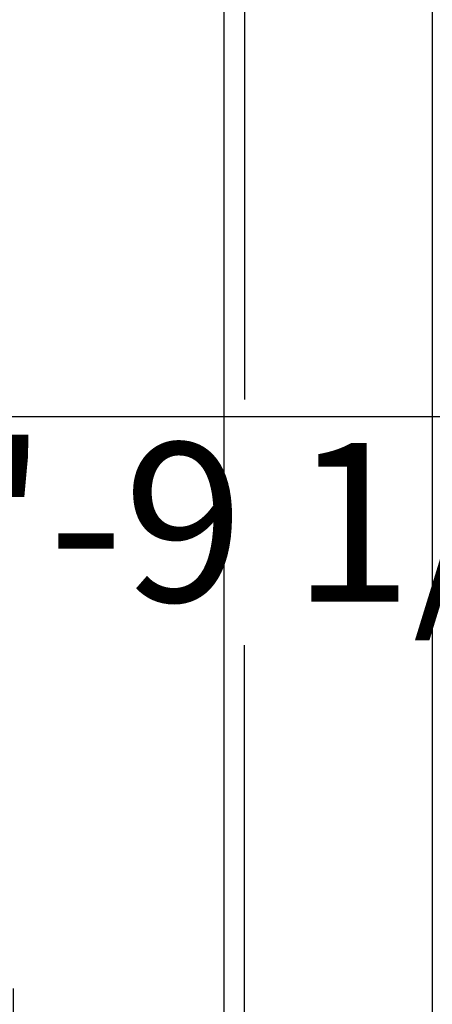
# Model space of a CAD drawing. Units: inches. Extents: x -26 to 385, y 12 to 697.
# Tile 8 of 13: x 264 to 285, y 165 to 215. Entities that reach past the tile are written whole.
import ezdxf

# ---------------------------------------------------------------- set-up
doc = ezdxf.new("R2010")
doc.units = ezdxf.units.IN
doc.header["$MEASUREMENT"] = 0
doc.layers.add('A-ANNO-DIMS', color=4, linetype='Continuous', lineweight=18)
doc.styles.get("Standard").update_dxf_attribs({"font": 'italic8.shx'})
doc.dimstyles.get("Standard").update_dxf_attribs({"dimtxt": 8, "dimasz": 0.18, "dimexe": 0.18, "dimexo": 0.0625, "dimgap": 0.09, "dimtad": 0, "dimtih": 1, "dimtoh": 1, "dimdec": 4, "dimzin": 0, "dimdsep": 46, "dimlunit": 3, "dimtxsty": 'Standard', "dimcen": 0.09, "dimclrd": 2, "dimclre": 3, "dimclrt": 6, "dimadec": 0, "dimazin": 0, "dimtfac": 1, "dimtdec": 4, "dimtofl": 0, "dimtmove": 0, "dimatfit": 3, "dimfxl": 1, "dimtolj": 1, "dimtzin": 0, "dimarcsym": 0})

# ---------------------------------------------------------------- blocks, each defined once
blk = doc.blocks.new('*D11')
at = {"layer": 'A-ANNO-DIMS', "color": 3, "lineweight": -2, "transparency": 16777216}
for p, q in [((285.56, 224.402), (274.992, 224.402)), ((285.56, 154.738), (274.992, 154.738))]:
    blk.add_line(p, q, dxfattribs=at)
at = {"layer": 'A-ANNO-DIMS', "color": 2, "lineweight": -2, "transparency": 16777216}
for p, q in [((275.172, 224.222), (275.172, 195.755)), ((275.172, 154.918), (275.172, 183.384))]:
    blk.add_line(p, q, dxfattribs=at)
at = {"layer": 'A-ANNO-DIMS', "color": 2, "transparency": 16777216}
for points in [[(275.142, 224.222), (275.202, 224.222), (275.172, 224.402)], [(275.142, 154.918), (275.202, 154.918), (275.172, 154.738)]]:
    blk.add_solid(points, dxfattribs=at)
at = {"layer": 'Defpoints', "color": 0, "transparency": 16777216}
for p in [(285.622, 224.402), (275.172, 154.738), (285.622, 154.738)]:
    blk.add_point(p, dxfattribs=at)
at = {"layer": 'A-ANNO-DIMS', "color": 6, "transparency": 16777216, "insert": (275.172, 189.57), "char_height": 8, "attachment_point": 5}
blk.add_mtext('\\A1;SOFA 5\'-9 1/2" TYP.', dxfattribs=at)
blk = doc.blocks.new('*D25')
at = {"layer": 'A-ANNO-DIMS', "color": 3, "lineweight": -2, "transparency": 16777216}
for p, q in [((284.629322, 368.316588), (284.629322, 23.949088)), ((320.629322, 368.316588), (320.629322, 23.949088))]:
    blk.add_line(p, q, dxfattribs=at)
at = {"layer": 'A-ANNO-DIMS', "color": 2, "lineweight": -2, "transparency": 16777216}
for p, q in [((284.449322, 24.129088), (284.269322, 24.129088)), ((320.809322, 24.129088), (320.989322, 24.129088))]:
    blk.add_line(p, q, dxfattribs=at)
at = {"layer": 'A-ANNO-DIMS', "color": 2, "transparency": 16777216}
for points in [[(284.449322, 24.159088), (284.449322, 24.099088), (284.629322, 24.129088)], [(320.809322, 24.159088), (320.809322, 24.099088), (320.629322, 24.129088)]]:
    blk.add_solid(points, dxfattribs=at)
at = {"layer": 'Defpoints', "color": 0, "transparency": 16777216}
for p in [(284.629322, 368.379088), (320.629322, 368.379088), (320.629322, 24.129088)]:
    blk.add_point(p, dxfattribs=at)
at = {"layer": 'A-ANNO-DIMS', "color": 6, "transparency": 16777216, "insert": (302.629322, 24.129088), "char_height": 8, "attachment_point": 5}
blk.add_mtext('\\A1;3\'-0"', dxfattribs=at)
blk = doc.blocks.new('*D28')
at = {"layer": 'A-ANNO-DIMS', "color": 3, "lineweight": -2, "transparency": 16777216}
for p, q in [((141.692, 194.903), (355.559, 194.903)), ((141.692, 158.903), (355.559, 158.903))]:
    blk.add_line(p, q, dxfattribs=at)
at = {"layer": 'A-ANNO-DIMS', "color": 2, "lineweight": -2, "transparency": 16777216}
for p, q in [((355.379, 194.723), (355.379, 181.755)), ((355.379, 159.083), (355.379, 172.052))]:
    blk.add_line(p, q, dxfattribs=at)
at = {"layer": 'A-ANNO-DIMS', "color": 2, "transparency": 16777216}
for points in [[(355.349, 194.723), (355.409, 194.723), (355.379, 194.903)], [(355.349, 159.083), (355.409, 159.083), (355.379, 158.903)]]:
    blk.add_solid(points, dxfattribs=at)
at = {"layer": 'Defpoints', "color": 0, "transparency": 16777216}
for p in [(141.629, 194.903), (355.379, 194.903), (141.629, 158.903)]:
    blk.add_point(p, dxfattribs=at)
at = {"layer": 'A-ANNO-DIMS', "color": 6, "transparency": 16777216, "insert": (355.379, 176.903), "char_height": 8, "attachment_point": 5}
blk.add_mtext('\\A1;3\'-0"', dxfattribs=at)
blk = doc.blocks.new('*D31')
at = {"layer": 'A-ANNO-DIMS', "color": 3, "lineweight": -2, "transparency": 16777216}
for p, q in [((239.888, 166.079), (239.888, 23.949)), ((263.51, 166.079), (263.51, 23.949))]:
    blk.add_line(p, q, dxfattribs=at)
at = {"layer": 'A-ANNO-DIMS', "color": 2, "lineweight": -2, "transparency": 16777216}
for p, q in [((240.068, 24.129), (263.33, 24.129)), ((263.51, 24.129), (263.69, 24.129))]:
    blk.add_line(p, q, dxfattribs=at)
at = {"layer": 'A-ANNO-DIMS', "color": 2, "transparency": 16777216}
for points in [[(240.068, 24.159), (240.068, 24.099), (239.888, 24.129)], [(263.33, 24.159), (263.33, 24.099), (263.51, 24.129)]]:
    blk.add_solid(points, dxfattribs=at)
at = {"layer": 'Defpoints', "color": 0, "transparency": 16777216}
for p in [(239.888, 166.141), (263.51, 166.141), (263.51, 24.129)]:
    blk.add_point(p, dxfattribs=at)
at = {"layer": 'A-ANNO-DIMS', "color": 6, "transparency": 16777216, "insert": (296.732, 24.129), "char_height": 8, "attachment_point": 5}
blk.add_mtext('\\A1;1\'-11 1/2"', dxfattribs=at)
blk = doc.blocks.new('*D35')
at = {"layer": 'A-ANNO-DIMS', "color": 3, "lineweight": -2, "transparency": 16777216}
for p, q in [((193.598, 147.942), (193.598, 684.809)), ((244.986, 147.942), (244.986, 684.809))]:
    blk.add_line(p, q, dxfattribs=at)
at = {"layer": 'A-ANNO-DIMS', "color": 2, "lineweight": -2, "transparency": 16777216}
for p, q in [((193.778, 684.629), (244.806, 684.629)), ((244.986, 684.629), (245.166, 684.629))]:
    blk.add_line(p, q, dxfattribs=at)
at = {"layer": 'A-ANNO-DIMS', "color": 2, "transparency": 16777216}
for points in [[(193.778, 684.659), (193.778, 684.599), (193.598, 684.629)], [(244.806, 684.659), (244.806, 684.599), (244.986, 684.629)]]:
    blk.add_solid(points, dxfattribs=at)
at = {"layer": 'Defpoints', "color": 0, "transparency": 16777216}
for p in [(244.986, 684.629), (193.598, 147.879), (244.986, 147.879)]:
    blk.add_point(p, dxfattribs=at)
at = {"layer": 'A-ANNO-DIMS', "color": 6, "transparency": 16777216, "insert": (278.398, 684.629), "char_height": 8, "attachment_point": 5}
blk.add_mtext('\\A1;4\'-3 1/2"', dxfattribs=at)
blk = doc.blocks.new('*D37')
at = {"layer": 'A-ANNO-DIMS', "color": 3, "lineweight": -2, "transparency": 16777216}
for p, q in [((223.549, 597.317), (223.549, 23.949)), ((257.22, 597.317), (257.22, 23.949))]:
    blk.add_line(p, q, dxfattribs=at)
at = {"layer": 'A-ANNO-DIMS', "color": 2, "lineweight": -2, "transparency": 16777216}
for p, q in [((223.729, 24.129), (257.04, 24.129)), ((257.22, 24.129), (257.4, 24.129))]:
    blk.add_line(p, q, dxfattribs=at)
at = {"layer": 'A-ANNO-DIMS', "color": 2, "transparency": 16777216}
for points in [[(223.729, 24.159), (223.729, 24.099), (223.549, 24.129)], [(257.04, 24.159), (257.04, 24.099), (257.22, 24.129)]]:
    blk.add_solid(points, dxfattribs=at)
at = {"layer": 'Defpoints', "color": 0, "transparency": 16777216}
for p in [(223.549, 597.379), (257.22, 597.379), (257.22, 24.129)]:
    blk.add_point(p, dxfattribs=at)
at = {"layer": 'A-ANNO-DIMS', "color": 6, "transparency": 16777216, "insert": (290.633, 24.129), "char_height": 8, "attachment_point": 5}
blk.add_mtext('\\A1;2\'-9 1/2"', dxfattribs=at)
blk = doc.blocks.new('*D42')
at = {"layer": 'A-ANNO-DIMS', "color": 3, "lineweight": -2, "transparency": 16777216}
for p, q in [((250.371, 518.992), (250.371, 23.949)), ((274.129, 518.992), (274.129, 23.949))]:
    blk.add_line(p, q, dxfattribs=at)
at = {"layer": 'A-ANNO-DIMS', "color": 2, "lineweight": -2, "transparency": 16777216}
for p, q in [((250.551, 24.129), (273.949, 24.129)), ((274.129, 24.129), (274.309, 24.129))]:
    blk.add_line(p, q, dxfattribs=at)
at = {"layer": 'A-ANNO-DIMS', "color": 2, "transparency": 16777216}
for points in [[(250.551, 24.159), (250.551, 24.099), (250.371, 24.129)], [(273.949, 24.159), (273.949, 24.099), (274.129, 24.129)]]:
    blk.add_solid(points, dxfattribs=at)
at = {"layer": 'Defpoints', "color": 0, "transparency": 16777216}
for p in [(250.371, 519.055), (274.129, 519.055), (274.129, 24.129)]:
    blk.add_point(p, dxfattribs=at)
at = {"layer": 'A-ANNO-DIMS', "color": 6, "transparency": 16777216, "insert": (292.304, 24.129), "char_height": 8, "attachment_point": 5}
blk.add_mtext('\\A1;2\'-0"', dxfattribs=at)
blk = doc.blocks.new('*D46')
at = {"layer": 'A-ANNO-DIMS', "color": 3, "lineweight": -2, "transparency": 16777216}
for p, q in [((224.595, 477.317), (224.595, 23.949)), ((284.629, 477.317), (284.629, 23.949))]:
    blk.add_line(p, q, dxfattribs=at)
at = {"layer": 'A-ANNO-DIMS', "color": 2, "lineweight": -2, "transparency": 16777216}
for p, q in [((224.775, 24.129), (236.617, 24.129)), ((284.449, 24.129), (272.607, 24.129))]:
    blk.add_line(p, q, dxfattribs=at)
at = {"layer": 'A-ANNO-DIMS', "color": 2, "transparency": 16777216}
for points in [[(224.775, 24.159), (224.775, 24.099), (224.595, 24.129)], [(284.449, 24.159), (284.449, 24.099), (284.629, 24.129)]]:
    blk.add_solid(points, dxfattribs=at)
at = {"layer": 'Defpoints', "color": 0, "transparency": 16777216}
for p in [(224.595, 477.379), (284.629, 477.379), (284.629, 24.129)]:
    blk.add_point(p, dxfattribs=at)
at = {"layer": 'A-ANNO-DIMS', "color": 6, "transparency": 16777216, "insert": (254.612, 24.129), "char_height": 8, "attachment_point": 5}
blk.add_mtext('\\A1;5\'-0"', dxfattribs=at)
blk = doc.blocks.new('*D50')
at = {"layer": 'A-ANNO-DIMS', "color": 3, "lineweight": -2, "transparency": 16777216}
for p, q in [((246.278, 401.871), (246.278, 23.949)), ((284.629, 398.317), (284.629, 23.949))]:
    blk.add_line(p, q, dxfattribs=at)
at = {"layer": 'A-ANNO-DIMS', "color": 2, "lineweight": -2, "transparency": 16777216}
for p, q in [((246.458, 24.129), (284.449, 24.129)), ((284.629, 24.129), (284.809, 24.129))]:
    blk.add_line(p, q, dxfattribs=at)
at = {"layer": 'A-ANNO-DIMS', "color": 2, "transparency": 16777216}
for points in [[(246.458, 24.159), (246.458, 24.099), (246.278, 24.129)], [(284.449, 24.159), (284.449, 24.099), (284.629, 24.129)]]:
    blk.add_solid(points, dxfattribs=at)
at = {"layer": 'Defpoints', "color": 0, "transparency": 16777216}
for p in [(246.278, 401.934), (284.629, 398.379), (284.629, 24.129)]:
    blk.add_point(p, dxfattribs=at)
at = {"layer": 'A-ANNO-DIMS', "color": 6, "transparency": 16777216, "insert": (318.042, 24.129), "char_height": 8, "attachment_point": 5}
blk.add_mtext('\\A1;3\'-2 1/2"', dxfattribs=at)

msp = doc.modelspace()

# ---------------------------------------------------------------- dimensions: what is measured, and where the dimension line sits
at = {"layer": 'A-ANNO-DIMS'}
for base, p1, p2, picture, middle in [((244.98557, 684.62909), (193.59818, 147.87909), (244.98557, 147.87909), '*D35', (278.39843, 684.62909)), ((257.21981, 24.12909), (223.54856, 597.37909), (257.21981, 597.37909), '*D37', (290.63267, 24.12909)), ((274.12932, 24.12909), (250.37102, 519.05498), (274.12932, 519.05498), '*D42', (292.30408, 24.12909)), ((284.62932, 24.12909), (224.59493, 477.37909), (284.62932, 477.37909), '*D46', (254.61213, 24.12909)), ((284.62932, 24.12909), (246.27828, 401.934), (284.62932, 398.37909), '*D50', (318.04218, 24.12909)), ((320.62932, 24.12909), (284.62932, 368.37909), (320.62932, 368.37909), '*D25', (302.62932, 24.12909)), ((263.50956, 24.12909), (239.88756, 166.14113), (263.50956, 166.14113), '*D31', (296.73194, 24.12909))]:
    dim = msp.add_linear_dim(base=base, p1=p1, p2=p2, dimstyle='Standard', override={"dimdec": 1, "dimlfac": 1, "dimrnd": 0, "dimzin": 1, "dimdsep": 46, "dimlunit": 4, "dimfrac": 2}, dxfattribs=at)
    dim.commit()
    dim.dimension.update_dxf_attribs({"geometry": picture, "text_midpoint": middle})
dim = msp.add_linear_dim(base=(275.17245, 154.73754), p1=(285.62207, 224.40165), p2=(285.62207, 154.73754), angle=270, text='SOFA <> TYP.', dimstyle='Standard', override={"dimdec": 1, "dimlfac": 1, "dimrnd": 0, "dimzin": 1, "dimdsep": 46, "dimlunit": 4, "dimfrac": 2}, dxfattribs=at)
dim.commit()
dim.dimension.update_dxf_attribs({"geometry": '*D11', "text_midpoint": (275.17245, 189.56959)})
dim = msp.add_linear_dim(base=(355.37932, 194.90341), p1=(141.62932, 158.90341), p2=(141.62932, 194.90341), angle=90, dimstyle='Standard', override={"dimdec": 1, "dimlfac": 1, "dimrnd": 0, "dimzin": 1, "dimdsep": 46, "dimlunit": 4, "dimfrac": 2}, dxfattribs=at)
dim.commit()
dim.dimension.update_dxf_attribs({"geometry": '*D28', "text_midpoint": (355.37932, 176.90341)})

doc.saveas('drawing.dxf')
